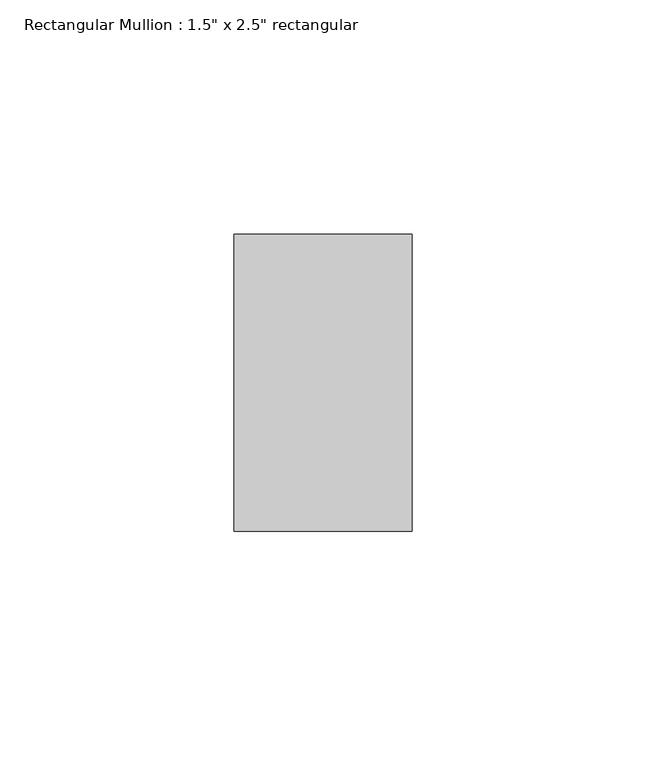
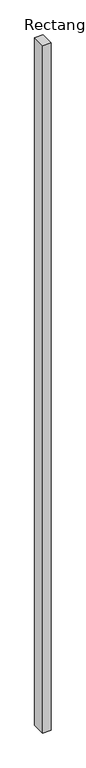
"""IFC4 building model written with IfcOpenShell, lengths in millimetres: member geometry."""

from ifc_helpers import new_model, si_unit, frame, origin, place, context, project, spatial, polyline, outline, extrude, source, transform, mapped, element, save


def member_235ee26f(model_context):
    return source(origin(), model_context, "Body", "SweptSolid", [
        extrude(outline(polyline([(0.0, 31.75), (0.0, -31.75), (-38.1, -31.75), (-38.1, 31.75), (0.0, 31.75)])), frame((0.0, 0.0, -3351.6454545), z_axis=(0.0, 0.0, 1.0), x_axis=(1.0, 0.0, 0.0)), (0.0, 0.0, 1.0), 3351.6454545),
    ])


if __name__ == "__main__":
    model = new_model("IFC4")
    model_context = context("Model", 3, world=origin())
    ifc_project = project(units=[si_unit("LENGTHUNIT", "METRE", prefix="MILLI")], contexts=[model_context])
    site = spatial("IfcSite", under=ifc_project)
    building = spatial("IfcBuilding", under=site)
    placement = place(None, origin())
    member_shape = member_235ee26f(model_context)
    element("IfcMember", 1, ObjectType="Rectangular Mullion : 1.5\" x 2.5\" rectangular", at=placement, inside=building, context=model_context, shape_type="MappedRepresentation", body=[
        mapped(member_shape, transform((0.0, 0.0, 0.0), x_axis=(1.0, 0.0, 0.0), y_axis=(0.0, 1.0, 0.0), z_axis=(0.0, 0.0, 1.0))),
    ])
    save(model, "model.ifc")

# Revit data of these elements
# Type "Rectangular Mullion : 1.5\" x 2.5\" rectangular"
#   built-in parameter 1007304 = 0.208333 (stored number, unit not read)
#   built-in parameter 1007301 = 0.0625 (stored number, unit not read)
#   built-in parameter 1007300 = 0.0625 (stored number, unit not read)
# Element 1 (IfcMember, "Rectangular Mullion : 1.5\" x 2.5\" rectangular")
#   Materials on its faces: "Aluminum"
# Materials
#   "Aluminum": class "Metal", colour RGB 247 247 247, transparency 0, Description = "Aluminum 6061", Cost = 0
